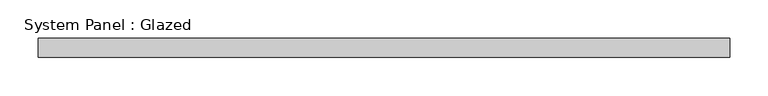
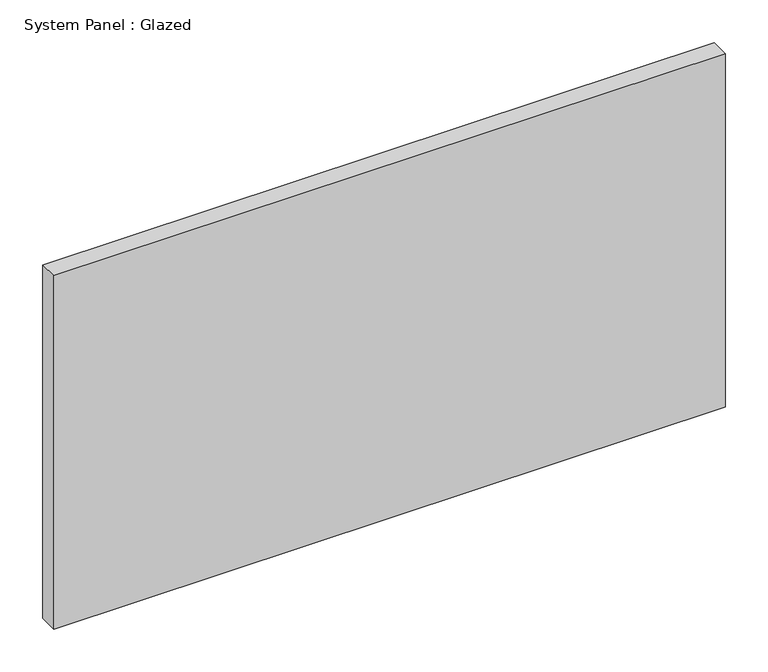
"""IFC4 building model written with IfcOpenShell, lengths in millimetres: plate geometry, System Panel : Glazed."""

from ifc_helpers import new_model, si_unit, origin, origin_with_axes, place, context, project, spatial, polyline, outline, extrude, source, transform, mapped, element, save


def system_panel_glazed_1607d5b8(model_context):
    return source(origin(), model_context, "Body", "SweptSolid", [
        extrude(outline(polyline([(451.25, 24.5), (-451.25, 24.5), (-451.25, 49.5), (451.25, 49.5), (451.25, 24.5)])), origin_with_axes(), (0.0, 0.0, 1.0), 502.5),
    ])


if __name__ == "__main__":
    model = new_model("IFC4")
    model_context = context("Model", 3, world=origin())
    ifc_project = project(units=[si_unit("LENGTHUNIT", "METRE", prefix="MILLI")], contexts=[model_context])
    site = spatial("IfcSite", under=ifc_project)
    building = spatial("IfcBuilding", under=site)
    placement = place(None, origin())
    system_panel_glazed_shape = system_panel_glazed_1607d5b8(model_context)
    element("IfcPlate", 1, ObjectType="System Panel : Glazed", at=placement, inside=building, context=model_context, shape_type="MappedRepresentation", body=[
        mapped(system_panel_glazed_shape, transform((0.0, 0.0, 0.0), x_axis=(1.0, 0.0, 0.0), y_axis=(0.0, 1.0, 0.0), z_axis=(0.0, 0.0, 1.0))),
    ])
    save(model, "model.ifc")

# Revit data of these elements
# Type "System Panel : Glazed"
#   Construction Type Id = "GSP4R"
#   Analytic Construction = "1/8 in Pilkington single glazing"
#   Visual Light Transmittance = 0.9
#   Solar Heat Gain Coefficient = 0.86
#   Heat Transfer Coefficient (U) = 6.7069 W/(m²·K)
#   Define Thermal Properties by = 1
# Element 1 (IfcPlate, "System Panel : Glazed")
#   Materials on its faces: "Glass"
# Materials
#   "Glass": class "Glass", colour RGB 245 245 243, transparency 1, Description = "Soda Lime Glass", Cost = 0
